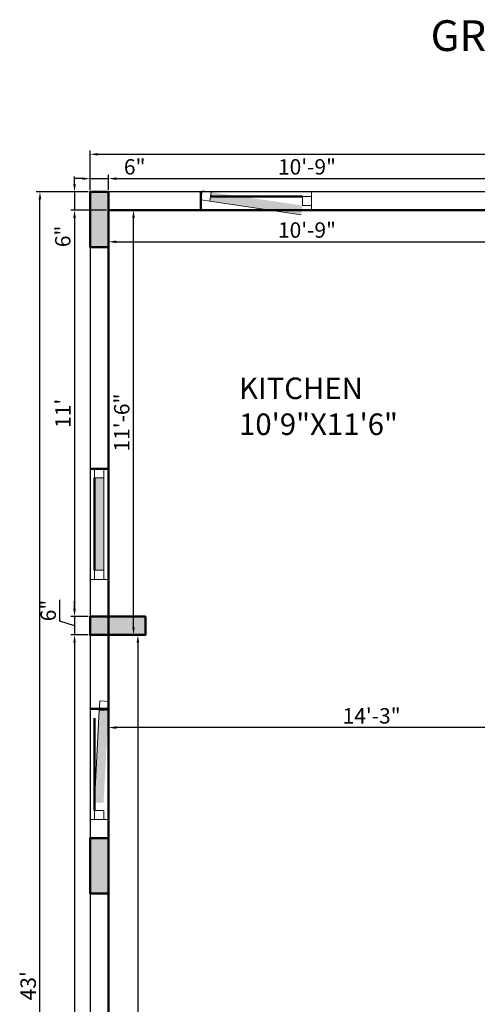
# Model space of a CAD drawing. Units: inches. Extents: x 3064 to 19385, y 846 to 15425.
# Tile 50 of 108: x 6020 to 6168, y 1132 to 1452. Entities that reach past the tile are written whole.
import ezdxf

# ---------------------------------------------------------------- set-up
doc = ezdxf.new("R2010")
doc.units = ezdxf.units.IN
for name, color, linetype, lineweight in [('A-ANNO-DIMS', 2, 'Continuous', 18), ('A-ANNO-TEXT', 7, 'Continuous', 25), ('A-AREA-IDEN', 3, 'Continuous', 18), ('A-COLS', 1, 'Continuous', 35), ('A-GLAZ', 4, 'Continuous', 18), ('A-WALL', 7, 'Continuous', 50), ('C-PROP', 6, 'Continuous', 25)]:
    doc.layers.add(name, color=color, linetype=linetype, lineweight=lineweight)
doc.styles.get("Standard").update_dxf_attribs({"font": 'arial.ttf'})
doc.dimstyles.new('ISO-25', dxfattribs={"dimtxt": 9, "dimasz": 2.5, "dimexe": 1.25, "dimexo": 0.625, "dimtad": 1, "dimdec": 1, "dimlunit": 3, "dimtxsty": 'Standard', "dimcen": 2.5, "dimadec": 0, "dimazin": 0, "dimtfac": 1, "dimtdec": 1, "dimtmove": 0, "dimatfit": 3, "dimfxl": 1, "dimarcsym": 0})

# ---------------------------------------------------------------- blocks, each defined once
blk = doc.blocks.new('*D140')
at = {"layer": 'A-ANNO-DIMS', "color": 0, "lineweight": -2, "transparency": 16777216}
for p, q in [((6042.49, 1396.96), (6042.49, 1401.84)), ((6048.49, 1396.96), (6048.49, 1401.84)), ((6039.99, 1400.59), (6037.49, 1400.59)), ((6042.49, 1400.59), (6048.49, 1400.59)), ((6050.99, 1400.59), (6060.52, 1400.59))]:
    blk.add_line(p, q, dxfattribs=at)
at = {"layer": 'A-ANNO-DIMS', "color": 0, "transparency": 16777216}
for points in [[(6039.99, 1401.01), (6039.99, 1400.18), (6042.49, 1400.59)], [(6050.99, 1401.01), (6050.99, 1400.18), (6048.49, 1400.59)]]:
    blk.add_solid(points, dxfattribs=at)
at = {"layer": 'Defpoints', "color": 0, "transparency": 16777216}
for p in [(6048.49, 1400.59), (6042.49, 1396.34), (6048.49, 1396.34)]:
    blk.add_point(p, dxfattribs=at)
at = {"layer": 'A-ANNO-DIMS', "color": 0, "transparency": 16777216, "insert": (6057, 1403.77), "char_height": 5, "attachment_point": 5}
blk.add_mtext('6"', dxfattribs=at)
blk = doc.blocks.new('*D141')
at = {"layer": 'A-ANNO-DIMS', "color": 0, "lineweight": -2, "transparency": 16777216}
for p, q in [((6048.49, 1396.96), (6048.49, 1401.84)), ((6177.49, 1396.96), (6177.49, 1401.84)), ((6050.99, 1400.59), (6174.99, 1400.59))]:
    blk.add_line(p, q, dxfattribs=at)
at = {"layer": 'A-ANNO-DIMS', "color": 0, "transparency": 16777216}
for points in [[(6050.99, 1401.01), (6050.99, 1400.18), (6048.49, 1400.59)], [(6174.99, 1401.01), (6174.99, 1400.18), (6177.49, 1400.59)]]:
    blk.add_solid(points, dxfattribs=at)
at = {"layer": 'Defpoints', "color": 0, "transparency": 16777216}
for p in [(6177.49, 1400.59), (6048.49, 1396.34), (6177.49, 1396.34)]:
    blk.add_point(p, dxfattribs=at)
at = {"layer": 'A-ANNO-DIMS', "color": 0, "transparency": 16777216, "insert": (6112.99, 1403.77), "char_height": 5, "attachment_point": 5}
blk.add_mtext('10\'-9"', dxfattribs=at)
blk = doc.blocks.new('*D145')
at = {"layer": 'A-ANNO-DIMS', "color": 0, "lineweight": -2, "transparency": 16777216}
for p, q in [((6037.46, 1398.84), (6037.46, 1401.34)), ((6041.87, 1396.34), (6036.21, 1396.34)), ((6037.46, 1396.34), (6037.46, 1390.34)), ((6047.87, 1390.34), (6036.21, 1390.34)), ((6037.46, 1387.84), (6037.46, 1378.32))]:
    blk.add_line(p, q, dxfattribs=at)
at = {"layer": 'A-ANNO-DIMS', "color": 0, "transparency": 16777216}
for points in [[(6037.05, 1398.84), (6037.88, 1398.84), (6037.46, 1396.34)], [(6037.05, 1387.84), (6037.88, 1387.84), (6037.46, 1390.34)]]:
    blk.add_solid(points, dxfattribs=at)
at = {"layer": 'Defpoints', "color": 0, "transparency": 16777216}
for p in [(6042.49, 1396.34), (6037.46, 1390.34), (6048.49, 1390.34)]:
    blk.add_point(p, dxfattribs=at)
at = {"layer": 'A-ANNO-DIMS', "color": 0, "transparency": 16777216, "insert": (6034.29, 1381.83), "char_height": 5, "attachment_point": 5, "rotation": 90}
blk.add_mtext('6"', dxfattribs=at)
blk = doc.blocks.new('*D146')
at = {"layer": 'A-ANNO-DIMS', "color": 0, "lineweight": -2, "transparency": 16777216}
for p, q in [((6047.87, 1390.34), (6036.21, 1390.34)), ((6037.46, 1387.84), (6037.46, 1260.84)), ((6041.87, 1258.34), (6036.21, 1258.34))]:
    blk.add_line(p, q, dxfattribs=at)
at = {"layer": 'A-ANNO-DIMS', "color": 0, "transparency": 16777216}
for points in [[(6037.05, 1387.84), (6037.88, 1387.84), (6037.46, 1390.34)], [(6037.05, 1260.84), (6037.88, 1260.84), (6037.46, 1258.34)]]:
    blk.add_solid(points, dxfattribs=at)
at = {"layer": 'Defpoints', "color": 0, "transparency": 16777216}
for p in [(6048.49, 1390.34), (6037.46, 1258.34), (6042.49, 1258.34)]:
    blk.add_point(p, dxfattribs=at)
at = {"layer": 'A-ANNO-DIMS', "color": 0, "transparency": 16777216, "insert": (6034.33, 1324.34), "char_height": 5, "attachment_point": 5, "rotation": 90}
blk.add_mtext("11'", dxfattribs=at)
blk = doc.blocks.new('*D147')
at = {"layer": 'A-ANNO-DIMS', "color": 0, "lineweight": -2, "transparency": 16777216}
for p, q in [((6032.72, 1256.76), (6032.72, 1263.79)), ((6037.46, 1260.84), (6037.46, 1263.34)), ((6041.87, 1258.34), (6036.21, 1258.34)), ((6037.46, 1258.34), (6037.46, 1252.34)), ((6037.46, 1258.34), (6037.46, 1252.34)), ((6037.46, 1255.34), (6032.72, 1256.76)), ((6041.87, 1252.34), (6036.21, 1252.34)), ((6037.46, 1249.84), (6037.46, 1247.34))]:
    blk.add_line(p, q, dxfattribs=at)
at = {"layer": 'A-ANNO-DIMS', "color": 0, "transparency": 16777216}
for points in [[(6037.05, 1260.84), (6037.88, 1260.84), (6037.46, 1258.34)], [(6037.05, 1249.84), (6037.88, 1249.84), (6037.46, 1252.34)]]:
    blk.add_solid(points, dxfattribs=at)
at = {"layer": 'Defpoints', "color": 0, "transparency": 16777216}
for p in [(6042.49, 1258.34), (6037.46, 1252.34), (6042.49, 1252.34)]:
    blk.add_point(p, dxfattribs=at)
at = {"layer": 'A-ANNO-DIMS', "color": 0, "transparency": 16777216, "insert": (6029.55, 1260.27), "char_height": 5, "attachment_point": 5, "rotation": 90}
blk.add_mtext('6"', dxfattribs=at)
blk = doc.blocks.new('*D136')
at = {"layer": 'A-ANNO-DIMS', "color": 0, "lineweight": -2, "transparency": 16777216}
for p, q in [((6041.87, 1252.34), (6036.21, 1252.34)), ((6037.46, 1249.84), (6037.46, 984.84)), ((6047.87, 982.34), (6036.21, 982.34))]:
    blk.add_line(p, q, dxfattribs=at)
at = {"layer": 'A-ANNO-DIMS', "color": 0, "transparency": 16777216}
for points in [[(6037.05, 1249.84), (6037.88, 1249.84), (6037.46, 1252.34)], [(6037.05, 984.84), (6037.88, 984.84), (6037.46, 982.34)]]:
    blk.add_solid(points, dxfattribs=at)
at = {"layer": 'Defpoints', "color": 0, "transparency": 16777216}
for p in [(6042.49, 1252.34), (6037.46, 982.34), (6048.49, 982.34)]:
    blk.add_point(p, dxfattribs=at)
at = {"layer": 'A-ANNO-DIMS', "color": 0, "transparency": 16777216, "insert": (6034.29, 1117.34), "char_height": 5, "attachment_point": 5, "rotation": 90}
blk.add_mtext('22\'-6"', dxfattribs=at)
blk = doc.blocks.new('*D110')
at = {"layer": 'A-ANNO-DIMS', "color": 0, "lineweight": -2, "transparency": 16777216}
for p, q in [((6041.87, 1396.34), (6024.98, 1396.34)), ((6026.23, 882.84), (6026.23, 1393.84)), ((6041.87, 880.34), (6024.98, 880.34))]:
    blk.add_line(p, q, dxfattribs=at)
at = {"layer": 'A-ANNO-DIMS', "color": 0, "transparency": 16777216}
for points in [[(6025.81, 1393.84), (6026.64, 1393.84), (6026.23, 1396.34)], [(6025.81, 882.84), (6026.64, 882.84), (6026.23, 880.34)]]:
    blk.add_solid(points, dxfattribs=at)
at = {"layer": 'Defpoints', "color": 0, "transparency": 16777216}
for p in [(6026.23, 1396.34), (6042.49, 1396.34), (6042.49, 880.34)]:
    blk.add_point(p, dxfattribs=at)
at = {"layer": 'A-ANNO-DIMS', "color": 0, "transparency": 16777216, "insert": (6023.05, 1138.34), "char_height": 5, "attachment_point": 5, "rotation": 90}
blk.add_mtext("43'", dxfattribs=at)
blk = doc.blocks.new('*D134')
at = {"layer": 'A-ANNO-DIMS', "color": 0, "lineweight": -2, "transparency": 16777216}
for p, q in [((6042.49, 1396.96), (6042.49, 1409.76)), ((6044.99, 1408.51), (6381.99, 1408.51)), ((6384.49, 1396.96), (6384.49, 1409.76))]:
    blk.add_line(p, q, dxfattribs=at)
at = {"layer": 'A-ANNO-DIMS', "color": 0, "transparency": 16777216}
for points in [[(6044.99, 1408.93), (6044.99, 1408.1), (6042.49, 1408.51)], [(6381.99, 1408.93), (6381.99, 1408.1), (6384.49, 1408.51)]]:
    blk.add_solid(points, dxfattribs=at)
at = {"layer": 'Defpoints', "color": 0, "transparency": 16777216}
for p in [(6384.49, 1408.51), (6042.49, 1396.34), (6384.49, 1396.34)]:
    blk.add_point(p, dxfattribs=at)
at = {"layer": 'A-ANNO-DIMS', "color": 0, "transparency": 16777216, "insert": (6213.49, 1411.69), "char_height": 5, "attachment_point": 5}
blk.add_mtext('28\'-6"', dxfattribs=at)
blk = doc.blocks.new('*D148')
at = {"layer": 'A-ANNO-DIMS', "color": 0, "lineweight": -2, "transparency": 16777216}
for p, q in [((6048.49, 1389.71), (6048.49, 1378.82)), ((6177.49, 1389.71), (6177.49, 1378.82)), ((6050.99, 1380.07), (6174.99, 1380.07))]:
    blk.add_line(p, q, dxfattribs=at)
at = {"layer": 'A-ANNO-DIMS', "color": 0, "transparency": 16777216}
for points in [[(6050.99, 1380.49), (6050.99, 1379.66), (6048.49, 1380.07)], [(6174.99, 1380.49), (6174.99, 1379.66), (6177.49, 1380.07)]]:
    blk.add_solid(points, dxfattribs=at)
at = {"layer": 'Defpoints', "color": 0, "transparency": 16777216}
for p in [(6048.49, 1390.34), (6177.49, 1390.34), (6177.49, 1380.07)]:
    blk.add_point(p, dxfattribs=at)
at = {"layer": 'A-ANNO-DIMS', "color": 0, "transparency": 16777216, "insert": (6112.99, 1383.25), "char_height": 5, "attachment_point": 5}
blk.add_mtext('10\'-9"', dxfattribs=at)
blk = doc.blocks.new('*D149')
at = {"layer": 'A-ANNO-DIMS', "color": 0, "lineweight": -2, "transparency": 16777216}
for p, q in [((6049.12, 1390.34), (6057.88, 1390.34)), ((6056.63, 1254.84), (6056.63, 1387.84)), ((6049.12, 1252.34), (6057.88, 1252.34))]:
    blk.add_line(p, q, dxfattribs=at)
at = {"layer": 'A-ANNO-DIMS', "color": 0, "transparency": 16777216}
for points in [[(6056.22, 1387.84), (6057.05, 1387.84), (6056.63, 1390.34)], [(6056.22, 1254.84), (6057.05, 1254.84), (6056.63, 1252.34)]]:
    blk.add_solid(points, dxfattribs=at)
at = {"layer": 'Defpoints', "color": 0, "transparency": 16777216}
for p in [(6048.49, 1390.34), (6056.63, 1390.34), (6048.49, 1252.34)]:
    blk.add_point(p, dxfattribs=at)
at = {"layer": 'A-ANNO-DIMS', "color": 0, "transparency": 16777216, "insert": (6053.45, 1321.34), "char_height": 5, "attachment_point": 5, "rotation": 90}
blk.add_mtext('11\'-6"', dxfattribs=at)
blk = doc.blocks.new('*D166')
at = {"layer": 'A-ANNO-DIMS', "color": 0, "lineweight": -2, "transparency": 16777216}
for p, q in [((6049.12, 1252.34), (6059.29, 1252.34)), ((6058.04, 1249.84), (6058.04, 984.84)), ((6049.12, 982.34), (6059.29, 982.34))]:
    blk.add_line(p, q, dxfattribs=at)
at = {"layer": 'A-ANNO-DIMS', "color": 0, "transparency": 16777216}
for points in [[(6057.63, 1249.84), (6058.46, 1249.84), (6058.04, 1252.34)], [(6057.63, 984.84), (6058.46, 984.84), (6058.04, 982.34)]]:
    blk.add_solid(points, dxfattribs=at)
at = {"layer": 'Defpoints', "color": 0, "transparency": 16777216}
for p in [(6048.49, 1252.34), (6048.49, 982.34), (6058.04, 982.34)]:
    blk.add_point(p, dxfattribs=at)
at = {"layer": 'A-ANNO-DIMS', "color": 0, "transparency": 16777216, "insert": (6054.87, 1117.34), "char_height": 5, "attachment_point": 5, "rotation": 90}
blk.add_mtext('22\'-6"', dxfattribs=at)
blk = doc.blocks.new('*D172')
at = {"layer": 'A-ANNO-DIMS', "color": 0, "lineweight": -2, "transparency": 16777216}
for p, q in [((6048.49, 1222.85), (6048.49, 1223.48)), ((6216.99, 1222.23), (6050.99, 1222.23)), ((6219.49, 1222.85), (6219.49, 1223.48))]:
    blk.add_line(p, q, dxfattribs=at)
at = {"layer": 'A-ANNO-DIMS', "color": 0, "transparency": 16777216}
for points in [[(6050.99, 1222.64), (6050.99, 1221.81), (6048.49, 1222.23)], [(6216.99, 1222.64), (6216.99, 1221.81), (6219.49, 1222.23)]]:
    blk.add_solid(points, dxfattribs=at)
at = {"layer": 'Defpoints', "color": 0, "transparency": 16777216}
for p in [(6048.49, 1222.23), (6048.49, 1222.23), (6219.49, 1222.23)]:
    blk.add_point(p, dxfattribs=at)
at = {"layer": 'A-ANNO-DIMS', "color": 0, "transparency": 16777216, "insert": (6133.99, 1225.4), "char_height": 5, "attachment_point": 5}
blk.add_mtext('14\'-3"', dxfattribs=at)
blk = doc.blocks.new('WIN-900-A')
h = blk.add_hatch(color=256)
h.dxf.hatch_style = 1
h.paths.add_polyline_path([(33, 0), (33, 3), (3, 3), (3, 0)])
blk.add_line((3, 0), (33, 0))
blk.add_lwpolyline([(3, 0), (0, 0), (0, 3), (3, 3)], close=True)
blk = doc.blocks.new('WIN-900')
blk.add_line((0, 0), (30, 0))
blk.add_lwpolyline([(30, 0), (30, 3), (33, 3), (33, 0)], close=True)

msp = doc.modelspace()

# ---------------------------------------------------------------- hatches: boundary and pattern name
at = {"layer": 'A-COLS'}
h = msp.add_hatch(color=256, dxfattribs=at)
h.dxf.hatch_style = 1
h.paths.add_polyline_path([(6042.49, 1378.34), (6048.49, 1378.34), (6048.49, 1396.34), (6042.49, 1396.34)])
h = msp.add_hatch(color=256, dxfattribs=at)
h.dxf.hatch_style = 1
h.paths.add_polyline_path([(6060.49, 1252.34), (6060.49, 1258.34), (6042.49, 1258.34), (6042.49, 1252.34)])
h = msp.add_hatch(color=256, dxfattribs=at)
h.dxf.hatch_style = 1
h.paths.add_polyline_path([(6042.49, 1168.34), (6048.49, 1168.34), (6048.49, 1186.34), (6042.49, 1186.34)])
at = {"layer": 'A-GLAZ'}
h = msp.add_hatch(color=256, dxfattribs=at)
h.dxf.hatch_style = 1
h.paths.add_polyline_path([(6043.99, 1273.34), (6046.99, 1273.34), (6046.99, 1303.34), (6043.99, 1303.34)])

# ---------------------------------------------------------------- linework, layer by layer
for p, q in [((6114.49, 1396.34), (6114.49, 1390.34)), ((6042.49, 1270.34), (6048.49, 1270.34)), ((6042.49, 1192.34), (6048.49, 1192.34))]:
    msp.add_line(p, q, dxfattribs=at)
for points in [[(6114.49, 1391.84), (6111.49, 1391.84), (6111.49, 1394.84), (6114.49, 1394.84)], [(6046.99, 1270.34), (6043.99, 1270.34), (6043.99, 1273.34), (6046.99, 1273.34)], [(6046.99, 1192.34), (6043.99, 1192.34), (6043.99, 1195.34), (6046.99, 1195.34)]]:
    msp.add_lwpolyline(points, close=True, dxfattribs=at)
at = {"layer": 'A-WALL'}
for p, q in [((6078.49, 1396.34), (6078.49, 1390.34)), ((6081.49, 1394.84), (6111.49, 1394.84)), ((6177.49, 1390.34), (6048.49, 1390.34)), ((6048.49, 1390.34), (6048.49, 982.34)), ((6042.49, 1306.34), (6048.49, 1306.34)), ((6043.99, 1303.34), (6043.99, 1273.34)), ((6048.49, 1252.34), (6060.49, 1252.34)), ((6042.49, 1228.34), (6048.49, 1228.34)), ((6043.99, 1225.34), (6043.99, 1195.34))]:
    msp.add_line(p, q, dxfattribs=at)
for points in [[(6048.49, 1378.34), (6048.49, 1396.34), (6042.49, 1396.34), (6042.49, 1378.34)], [(6060.49, 1258.34), (6042.49, 1258.34), (6042.49, 1252.34), (6060.49, 1252.34)], [(6048.49, 1168.34), (6048.49, 1186.34), (6042.49, 1186.34), (6042.49, 1168.34)]]:
    msp.add_lwpolyline(points, close=True, dxfattribs=at)
at = {"layer": 'C-PROP'}
for p, q in [((6384.49, 1396.34), (6042.49, 1396.34)), ((6042.49, 1396.34), (6042.49, 880.34))]:
    msp.add_line(p, q, dxfattribs=at)

# ---------------------------------------------------------------- block references
at = {"layer": 'A-GLAZ'}
for name, p, rotation in [('WIN-900-A', (6078.48, 1393.67), 351.6350998303229), ('WIN-900', (6046.99, 1273.34), 90.00000000000036), ('WIN-900-A', (6045.67, 1230.88), 266.9173551180347)]:
    msp.add_blockref(name, p, dxfattribs=dict(at, rotation=rotation))

# ---------------------------------------------------------------- texts
at = {"layer": 'A-ANNO-TEXT', "insert": (6153.16, 1452.06), "char_height": 10, "attachment_point": 1}
msp.add_mtext_dynamic_manual_height_columns('GROUND FLOOR PLAN', width=200.9739, gutter_width=12.5, heights=[0], dxfattribs=at)
at = {"layer": 'A-AREA-IDEN', "insert": (6090.91, 1335.96), "char_height": 7, "attachment_point": 1}
msp.add_mtext_dynamic_manual_height_columns('KITCHEN\\P10\'9"X11\'6"', width=67.5924, gutter_width=12.5, heights=[0], dxfattribs=at)

# ---------------------------------------------------------------- dimensions: what is measured, and where the dimension line sits
at = {"layer": 'A-ANNO-DIMS'}
for base, p1, p2, override, picture, middle in [((6384.49, 1408.51), (6042.49, 1396.34), (6384.49, 1396.34), {"dimtxt": 5, "dimclrd": 0, "dimclre": 0, "dimclrt": 0}, '*D134', (6213.49, 1411.69)), ((6048.49, 1400.59), (6042.49, 1396.34), (6048.49, 1396.34), {"dimtxt": 5, "dimclrd": 0, "dimclre": 0, "dimclrt": 0}, '*D140', (6057, 1403.77)), ((6177.49, 1400.59), (6048.49, 1396.34), (6177.49, 1396.34), {"dimtxt": 5, "dimclrd": 0, "dimclre": 0, "dimclrt": 0, "dimtmove": 1}, '*D141', (6112.99, 1403.77)), ((6177.49, 1380.07), (6048.49, 1390.34), (6177.49, 1390.34), {"dimtxt": 5, "dimclrd": 0, "dimclre": 0, "dimclrt": 0}, '*D148', (6112.99, 1383.25)), ((6048.49, 1222.23), (6219.49, 1222.23), (6048.49, 1222.23), {"dimtxt": 5, "dimclrd": 0, "dimclre": 0, "dimclrt": 0}, '*D172', (6133.99, 1225.4))]:
    dim = msp.add_linear_dim(base=base, p1=p1, p2=p2, dimstyle='ISO-25', override=override, dxfattribs=at)
    dim.commit()
    dim.dimension.update_dxf_attribs({"geometry": picture, "text_midpoint": middle})
for base, p1, p2, override, picture, middle in [((6037.46, 1390.34), (6042.49, 1396.34), (6048.49, 1390.34), {"dimtxt": 5, "dimclrd": 0, "dimclre": 0, "dimclrt": 0}, '*D145', (6034.29, 1381.83)), ((6026.23, 1396.34), (6042.49, 880.34), (6042.49, 1396.34), {"dimtxt": 5, "dimclrd": 0, "dimclre": 0, "dimclrt": 0}, '*D110', (6023.05, 1138.34)), ((6037.46, 1258.34), (6048.49, 1390.34), (6042.49, 1258.34), {"dimtxt": 5, "dimclrd": 0, "dimclre": 0, "dimclrt": 0, "dimtmove": 1}, '*D146', (6034.33, 1324.34)), ((6056.63, 1390.34), (6048.49, 1252.34), (6048.49, 1390.34), {"dimtxt": 5, "dimclrd": 0, "dimclre": 0, "dimclrt": 0}, '*D149', (6053.45, 1321.34)), ((6037.46, 1252.34), (6042.49, 1258.34), (6042.49, 1252.34), {"dimtxt": 5, "dimclrd": 0, "dimclre": 0, "dimclrt": 0, "dimtmove": 1}, '*D147', (6029.55, 1257.39)), ((6037.46, 982.34), (6042.49, 1252.34), (6048.49, 982.34), {"dimtxt": 5, "dimclrd": 0, "dimclre": 0, "dimclrt": 0, "dimtmove": 1}, '*D136', (6034.29, 1117.34)), ((6058.04, 982.34), (6048.49, 1252.34), (6048.49, 982.34), {"dimtxt": 5, "dimclrd": 0, "dimclre": 0, "dimclrt": 0}, '*D166', (6054.87, 1117.34))]:
    dim = msp.add_linear_dim(base=base, p1=p1, p2=p2, angle=90, dimstyle='ISO-25', override=override, dxfattribs=at)
    dim.commit()
    dim.dimension.update_dxf_attribs({"geometry": picture, "text_midpoint": middle})

doc.saveas('drawing.dxf')
